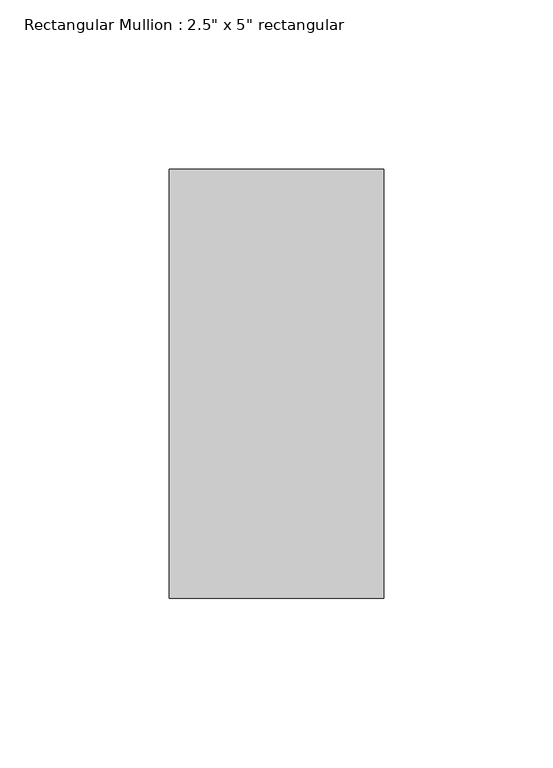
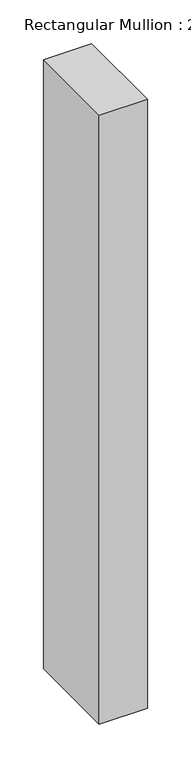
"""IFC4 building model written with IfcOpenShell, lengths in millimetres: member geometry."""

from ifc_helpers import new_model, si_unit, frame, origin, place, context, project, spatial, polyline, outline, extrude, source, transform, mapped, element, save


def member_ceca9e34(model_context):
    return source(origin(), model_context, "Body", "SweptSolid", [
        extrude(outline(polyline([(0.0, 63.5), (0.0, -63.5), (-63.5, -63.5), (-63.5, 63.5), (0.0, 63.5)])), frame((0.0, 0.0, -848.7833333), z_axis=(0.0, 0.0, 1.0), x_axis=(1.0, 0.0, 0.0)), (0.0, 0.0, 1.0), 848.7833333),
    ])


if __name__ == "__main__":
    model = new_model("IFC4")
    model_context = context("Model", 3, world=origin())
    ifc_project = project(units=[si_unit("LENGTHUNIT", "METRE", prefix="MILLI")], contexts=[model_context])
    site = spatial("IfcSite", under=ifc_project)
    building = spatial("IfcBuilding", under=site)
    placement = place(None, origin())
    member_shape = member_ceca9e34(model_context)
    element("IfcMember", 1, ObjectType="Rectangular Mullion : 2.5\" x 5\" rectangular", at=placement, inside=building, context=model_context, shape_type="MappedRepresentation", body=[
        mapped(member_shape, transform((0.0, 0.0, 0.0), x_axis=(1.0, 0.0, 0.0), y_axis=(0.0, 1.0, 0.0), z_axis=(0.0, 0.0, 1.0))),
    ])
    save(model, "model.ifc")

# Revit data of these elements
# Type "Rectangular Mullion : 2.5\" x 5\" rectangular"
#   built-in parameter 1007304 = 0.416667 (stored number, unit not read)
#   built-in parameter 1007301 = 0.104167 (stored number, unit not read)
#   built-in parameter 1007300 = 0.104167 (stored number, unit not read)
# Element 1 (IfcMember, "Rectangular Mullion : 2.5\" x 5\" rectangular")
#   Materials on its faces: "Aluminum"
# Materials
#   "Aluminum": class "Metal", colour RGB 247 247 247, transparency 0, Description = "Aluminum 6061", Cost = 0
